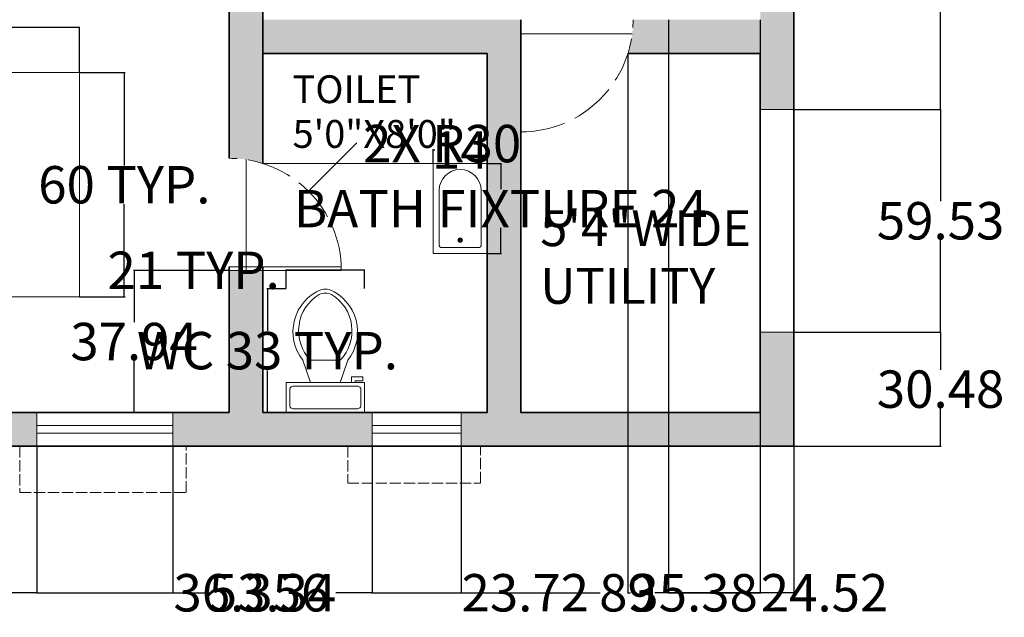
# Model space of a CAD drawing. Units: inches. Extents: x 143 to 746, y -392 to 145.
# Tile 4 of 6: x 473 to 736, y -392 to -233. Entities that reach past the tile are written whole.
import ezdxf

# ---------------------------------------------------------------- set-up
doc = ezdxf.new("R2010")
doc.units = ezdxf.units.IN
doc.header["$MEASUREMENT"] = 0
doc.linetypes.add('ACAD_ISO02W100', pattern=[15, 12, -3])
for name, color, linetype, lineweight in [('A-ANNO-DIMS', 2, 'Continuous', 18), ('A-AREA-IDEN', 7, 'Continuous', 20), ('A-DOOR', 3, 'Continuous', 18), ('A-DOOR-SWNG', 3, 'ACAD_ISO02W100', 13), ('A-FLOR-FIXT', 9, 'Continuous', 18), ('A-FURN', 8, 'Continuous', 18), ('A-GLAZ', 4, 'Continuous', 18), ('A-GLAZ-OVHD', 4, 'ACAD_ISO02W100', 13), ('A-WALL', 7, 'Continuous', 35)]:
    doc.layers.add(name, color=color, linetype=linetype, lineweight=lineweight)
doc.layers.add('A-WALL-PATT', color=252, linetype='Continuous', lineweight=13, true_color=0x939598)
doc.styles.get("Standard").update_dxf_attribs({"font": 'arial.ttf'})
doc.dimstyles.get("Standard").update_dxf_attribs({"dimtxt": 10, "dimasz": 0.18, "dimexe": 0.18, "dimexo": 0.0625, "dimgap": 0.09, "dimtad": 0, "dimtih": 1, "dimtoh": 1, "dimdec": 0, "dimzin": 0, "dimdsep": 46, "dimlunit": 3, "dimtxsty": 'Standard', "dimcen": 0.09, "dimadec": 0, "dimazin": 0, "dimtfac": 1, "dimtdec": 0, "dimtofl": 0, "dimtmove": 0, "dimatfit": 3, "dimfxl": 1, "dimtolj": 1, "dimtzin": 0, "dimarcsym": 0})

# ---------------------------------------------------------------- blocks, each defined once
blk = doc.blocks.new('Toilet - top')
for p, q in [((9.5, -6), (9.5, -2)), ((-10, -8.5), (-8, -8.5)), ((-10, -9.5), (-10, -8.5)), ((-7, -9.5), (-10, -9.5)), ((-8, -8.5), (-8, -8)), ((-7, -8), (-7, -9.5)), ((-4, -8), (-6, -14)), ((4, -8), (6, -14)), ((4, -14), (-4, -14))]:
    blk.add_line(p, q)
blk.add_lwpolyline([(10.5, -8), (10.5, 0), (-10.5, 0), (-10.5, -8)], close=True)
for points in [[(-9.5, -2), (-9.5, -6)], [(8.5, -1), (-8.5, -1)], [(-8.5, -7), (8.5, -7)]]:
    blk.add_lwpolyline(points)
for centre, radius, start, end in [((-8.62, -1.88), 0.884, 81.8699, 188.1301), ((8.62, -1.88), 0.884, 351.8699, 98.1301), ((-8.62, -6.12), 0.884, 171.8699, 278.1301), ((8.62, -6.12), 0.884, 261.8699, 8.1301), ((3.52, -21.58), 12.17, 141.4691, 247.9714), ((4.2, -21.82), 11.33, 136.3677, 238.9468), ((-3.52, -21.58), 12.17, 292.0284, 38.5307), ((-4.2, -21.82), 11.33, 301.053, 43.6321), ((0, -27.88), 4, 245.7318, 294.2682), ((0, -29), 4, 254.8605, 285.1395)]:
    blk.add_arc(centre, radius, start, end)
blk = doc.blocks.new('Bath Tub - 26 x 60 in.')
for p, q in [((8, -18), (10, -18)), ((9, -17), (9, -19))]:
    blk.add_line(p, q)
blk.add_lwpolyline([(0, -36), (0, 0), (60, 0), (60, -36)], close=True)
for points in [[(4, -30), (4, -6)], [(6, -4), (42, -4)], [(42, -32), (6, -32)]]:
    blk.add_lwpolyline(points)
for radius in [1.5, 1]:
    blk.add_circle((9, -18), radius)
for centre, radius, start, end in [((5.75, -5.75), 1.77, 81.8699, 188.1301), ((42, -18), 14, 270, 90), ((5.75, -30.25), 1.77, 171.8699, 278.1301)]:
    blk.add_arc(centre, radius, start, end)
blk = doc.blocks.new('Bed - Queen')
for p, q in [((0, -80.00003), (0, 0)), ((0, 0), (59.99999, 0)), ((59.99999, 0), (59.99999, -80.00003)), ((7.99999, -1.2), (28.79998, -1.2)), ((7.99999, -14.4), (7.99999, -1.2)), ((28.79998, -1.2), (28.79998, -14.4)), ((31.19999, -1.2), (51.99999, -1.2)), ((31.19999, -14.4), (31.19999, -1.2)), ((51.99999, -1.2), (51.99999, -16.4)), ((0, -14.4), (44.8, -14.4)), ((59.99999, -29.6), (44.8, -14.4)), ((44.8, -14.4), (44.8, -29.6)), ((44.8, -16.8), (0, -16.8)), ((51.99999, -16.4), (46.79936, -16.4)), ((44.8, -29.6), (59.99999, -29.6)), ((59.99999, -80.00003), (0, -80.00003))]:
    blk.add_line(p, q)
blk = doc.blocks.new('*D12')
at = {"layer": 'A-ANNO-DIMS', "color": 0, "lineweight": -2, "transparency": 16777216}
for p, q in [((369.19, -220.67), (369.19, -225.34)), ((399.54, -220.67), (399.54, -225.34)), ((369.37, -225.16), (399.36, -225.16)), ((399.54, -225.16), (399.72, -225.16))]:
    blk.add_line(p, q, dxfattribs=at)
at = {"layer": 'A-ANNO-DIMS', "color": 0, "transparency": 16777216}
for points in [[(369.37, -225.13), (369.37, -225.19), (369.19, -225.16)], [(399.36, -225.13), (399.36, -225.19), (399.54, -225.16)]]:
    blk.add_solid(points, dxfattribs=at)
at = {"layer": 'Defpoints', "color": 0, "transparency": 16777216}
for p in [(369.19, -220.61), (399.54, -220.61), (399.54, -225.16)]:
    blk.add_point(p, dxfattribs=at)
at = {"layer": 'A-ANNO-DIMS', "color": 0, "transparency": 16777216, "insert": (459.12, -225.16), "char_height": 10, "attachment_point": 5}
blk.add_mtext('\\A1;BATH FIXTURE 30', dxfattribs=at)
blk = doc.blocks.new('*D14')
at = {"layer": 'A-ANNO-DIMS', "color": 0, "lineweight": -2, "transparency": 16777216}
for p, q in [((597.6, -271.05), (601.33, -271.05)), ((601.15, -271.23), (601.15, -277.9)), ((601.15, -294.96), (601.15, -288.29)), ((597.6, -295.14), (601.33, -295.14))]:
    blk.add_line(p, q, dxfattribs=at)
at = {"layer": 'A-ANNO-DIMS', "color": 0, "transparency": 16777216}
for points in [[(601.12, -271.23), (601.18, -271.23), (601.15, -271.05)], [(601.12, -294.96), (601.18, -294.96), (601.15, -295.14)]]:
    blk.add_solid(points, dxfattribs=at)
at = {"layer": 'Defpoints', "color": 0, "transparency": 16777216}
for p in [(597.54, -271.05), (601.15, -271.05), (597.54, -295.14)]:
    blk.add_point(p, dxfattribs=at)
at = {"layer": 'A-ANNO-DIMS', "color": 0, "transparency": 16777216, "insert": (601.15, -283.1), "char_height": 10, "attachment_point": 5}
blk.add_mtext('\\A1;BATH FIXTURE 24', dxfattribs=at)
blk = doc.blocks.new('*D15')
at = {"layer": 'A-ANNO-DIMS', "color": 0, "lineweight": -2, "transparency": 16777216}
for p, q in [((583.08, -270.99), (583.08, -267.25)), ((583.26, -267.43), (583.55, -267.43)), ((597.36, -267.43), (597.07, -267.43)), ((597.54, -270.99), (597.54, -267.25))]:
    blk.add_line(p, q, dxfattribs=at)
at = {"layer": 'A-ANNO-DIMS', "color": 0, "transparency": 16777216}
for points in [[(583.26, -267.4), (583.26, -267.46), (583.08, -267.43)], [(597.36, -267.4), (597.36, -267.46), (597.54, -267.43)]]:
    blk.add_solid(points, dxfattribs=at)
at = {"layer": 'Defpoints', "color": 0, "transparency": 16777216}
for p in [(583.08, -267.43), (583.08, -271.05), (597.54, -271.05)]:
    blk.add_point(p, dxfattribs=at)
at = {"layer": 'A-ANNO-DIMS', "color": 0, "transparency": 16777216, "insert": (590.31, -267.43), "char_height": 10, "attachment_point": 5}
blk.add_mtext('\\A1;14', dxfattribs=at)
blk = doc.blocks.new('*D22')
at = {"layer": 'A-ANNO-DIMS', "color": 0, "lineweight": -2, "transparency": 16777216}
for p, q in [((543.7, -304.56), (538.62, -304.56)), ((538.8, -304.74), (538.8, -315.82)), ((538.8, -337.43), (538.8, -326.35)), ((543.7, -337.61), (538.62, -337.61))]:
    blk.add_line(p, q, dxfattribs=at)
at = {"layer": 'A-ANNO-DIMS', "color": 0, "transparency": 16777216}
for points in [[(538.77, -304.74), (538.83, -304.74), (538.8, -304.56)], [(538.77, -337.43), (538.83, -337.43), (538.8, -337.61)]]:
    blk.add_solid(points, dxfattribs=at)
at = {"layer": 'Defpoints', "color": 0, "transparency": 16777216}
for p in [(543.76, -304.56), (538.8, -337.61), (543.76, -337.61)]:
    blk.add_point(p, dxfattribs=at)
at = {"layer": 'A-ANNO-DIMS', "color": 0, "transparency": 16777216, "insert": (538.8, -321.08), "char_height": 10, "attachment_point": 5}
blk.add_mtext('\\A1;WC 33 TYP.', dxfattribs=at)
blk = doc.blocks.new('*D23')
at = {"layer": 'A-ANNO-DIMS', "color": 0, "lineweight": -2, "transparency": 16777216}
for p, q in [((543.76, -299.6), (543.58, -299.6)), ((543.76, -304.5), (543.76, -299.42)), ((564.58, -299.6), (543.94, -299.6)), ((564.76, -304.5), (564.76, -299.42))]:
    blk.add_line(p, q, dxfattribs=at)
at = {"layer": 'A-ANNO-DIMS', "color": 0, "transparency": 16777216}
for points in [[(543.94, -299.57), (543.94, -299.63), (543.76, -299.6)], [(564.58, -299.57), (564.58, -299.63), (564.76, -299.6)]]:
    blk.add_solid(points, dxfattribs=at)
at = {"layer": 'Defpoints', "color": 0, "transparency": 16777216}
for p in [(543.76, -299.6), (543.76, -304.56), (564.76, -304.56)]:
    blk.add_point(p, dxfattribs=at)
at = {"layer": 'A-ANNO-DIMS', "color": 0, "transparency": 16777216, "insert": (519.07, -299.6), "char_height": 10, "attachment_point": 5}
blk.add_mtext('\\A1;21 TYP.', dxfattribs=at)
blk = doc.blocks.new('*D24')
at = {"layer": 'A-ANNO-DIMS', "color": 0, "lineweight": -2, "transparency": 16777216}
for p, q in [((408.54, -234.73), (408.36, -234.73)), ((408.54, -246.67), (408.54, -234.55)), ((488.36, -234.73), (408.72, -234.73)), ((488.54, -246.67), (488.54, -234.55))]:
    blk.add_line(p, q, dxfattribs=at)
at = {"layer": 'A-ANNO-DIMS', "color": 0, "transparency": 16777216}
for points in [[(408.72, -234.7), (408.72, -234.76), (408.54, -234.73)], [(488.36, -234.7), (488.36, -234.76), (488.54, -234.73)]]:
    blk.add_solid(points, dxfattribs=at)
at = {"layer": 'Defpoints', "color": 0, "transparency": 16777216}
for p in [(408.54, -234.73), (408.54, -246.73), (488.54, -246.73)]:
    blk.add_point(p, dxfattribs=at)
at = {"layer": 'A-ANNO-DIMS', "color": 0, "transparency": 16777216, "insert": (340.86, -234.73), "char_height": 10, "attachment_point": 5}
blk.add_mtext('\\A1;QUEEN BED 80 TYP.', dxfattribs=at)
blk = doc.blocks.new('*D25')
at = {"layer": 'A-ANNO-DIMS', "color": 0, "lineweight": -2, "transparency": 16777216}
for p, q in [((488.6, -246.73), (500.72, -246.73)), ((500.54, -246.91), (500.54, -271.54)), ((500.54, -306.55), (500.54, -281.93)), ((488.6, -306.73), (500.72, -306.73))]:
    blk.add_line(p, q, dxfattribs=at)
at = {"layer": 'A-ANNO-DIMS', "color": 0, "transparency": 16777216}
for points in [[(500.51, -246.91), (500.57, -246.91), (500.54, -246.73)], [(500.51, -306.55), (500.57, -306.55), (500.54, -306.73)]]:
    blk.add_solid(points, dxfattribs=at)
at = {"layer": 'Defpoints', "color": 0, "transparency": 16777216}
for p in [(488.54, -246.73), (500.54, -246.73), (488.54, -306.73)]:
    blk.add_point(p, dxfattribs=at)
at = {"layer": 'A-ANNO-DIMS', "color": 0, "transparency": 16777216, "insert": (500.54, -276.73), "char_height": 10, "attachment_point": 5}
blk.add_mtext('\\A1;60 TYP.', dxfattribs=at)
blk = doc.blocks.new('*D38')
at = {"layer": 'A-ANNO-DIMS', "color": 0, "lineweight": -2, "transparency": 16777216}
for p, q in [((388.66, -346.67), (388.66, -385.98)), ((477.13, -346.67), (477.13, -385.98)), ((388.84, -385.8), (415.92, -385.8)), ((476.95, -385.8), (449.86, -385.8))]:
    blk.add_line(p, q, dxfattribs=at)
at = {"layer": 'A-ANNO-DIMS', "color": 0, "transparency": 16777216}
for points in [[(388.84, -385.77), (388.84, -385.83), (388.66, -385.8)], [(476.95, -385.77), (476.95, -385.83), (477.13, -385.8)]]:
    blk.add_solid(points, dxfattribs=at)
at = {"layer": 'Defpoints', "color": 0, "transparency": 16777216}
for p in [(388.66, -346.61), (477.13, -346.61), (477.13, -385.8)]:
    blk.add_point(p, dxfattribs=at)
at = {"layer": 'A-ANNO-DIMS', "color": 0, "transparency": 16777216, "insert": (432.89, -385.8), "char_height": 10, "attachment_point": 5}
blk.add_mtext('\\A1;88.47', dxfattribs=at)
blk = doc.blocks.new('*D39')
at = {"layer": 'A-ANNO-DIMS', "color": 0, "lineweight": -2, "transparency": 16777216}
for p, q in [((477.13, -346.67), (477.13, -385.98)), ((513.48, -346.67), (513.48, -385.98)), ((477.31, -385.8), (513.3, -385.8)), ((513.48, -385.8), (513.66, -385.8))]:
    blk.add_line(p, q, dxfattribs=at)
at = {"layer": 'A-ANNO-DIMS', "color": 0, "transparency": 16777216}
for points in [[(477.31, -385.77), (477.31, -385.83), (477.13, -385.8)], [(513.3, -385.77), (513.3, -385.83), (513.48, -385.8)]]:
    blk.add_solid(points, dxfattribs=at)
at = {"layer": 'Defpoints', "color": 0, "transparency": 16777216}
for p in [(477.13, -346.61), (513.48, -346.61), (513.48, -385.8)]:
    blk.add_point(p, dxfattribs=at)
at = {"layer": 'A-ANNO-DIMS', "color": 0, "transparency": 16777216, "insert": (534.5, -385.8), "char_height": 10, "attachment_point": 5}
blk.add_mtext('\\A1;36.356', dxfattribs=at)
blk = doc.blocks.new('*D40')
at = {"layer": 'A-ANNO-DIMS', "color": 0, "lineweight": -2, "transparency": 16777216}
for p, q in [((513.48, -346.67), (513.48, -385.98)), ((566.83, -346.67), (566.83, -385.98)), ((513.66, -385.8), (523.21, -385.8)), ((566.65, -385.8), (557.1, -385.8))]:
    blk.add_line(p, q, dxfattribs=at)
at = {"layer": 'A-ANNO-DIMS', "color": 0, "transparency": 16777216}
for points in [[(513.66, -385.77), (513.66, -385.83), (513.48, -385.8)], [(566.65, -385.77), (566.65, -385.83), (566.83, -385.8)]]:
    blk.add_solid(points, dxfattribs=at)
at = {"layer": 'Defpoints', "color": 0, "transparency": 16777216}
for p in [(513.48, -346.61), (566.83, -346.61), (566.83, -385.8)]:
    blk.add_point(p, dxfattribs=at)
at = {"layer": 'A-ANNO-DIMS', "color": 0, "transparency": 16777216, "insert": (540.15, -385.8), "char_height": 10, "attachment_point": 5}
blk.add_mtext('\\A1;53.34', dxfattribs=at)
blk = doc.blocks.new('*D41')
at = {"layer": 'A-ANNO-DIMS', "color": 0, "lineweight": -2, "transparency": 16777216}
for p, q in [((566.83, -346.67), (566.83, -385.98)), ((590.54, -346.67), (590.54, -385.98)), ((567.01, -385.8), (590.36, -385.8)), ((590.54, -385.8), (590.72, -385.8))]:
    blk.add_line(p, q, dxfattribs=at)
at = {"layer": 'A-ANNO-DIMS', "color": 0, "transparency": 16777216}
for points in [[(567.01, -385.77), (567.01, -385.83), (566.83, -385.8)], [(590.36, -385.77), (590.36, -385.83), (590.54, -385.8)]]:
    blk.add_solid(points, dxfattribs=at)
at = {"layer": 'Defpoints', "color": 0, "transparency": 16777216}
for p in [(566.83, -346.61), (590.54, -346.61), (590.54, -385.8)]:
    blk.add_point(p, dxfattribs=at)
at = {"layer": 'A-ANNO-DIMS', "color": 0, "transparency": 16777216, "insert": (607.72, -385.8), "char_height": 10, "attachment_point": 5}
blk.add_mtext('\\A1;23.72', dxfattribs=at)
blk = doc.blocks.new('*D42')
at = {"layer": 'A-ANNO-DIMS', "color": 0, "lineweight": -2, "transparency": 16777216}
for p, q in [((590.54, -346.67), (590.54, -385.98)), ((679.54, -346.67), (679.54, -385.98)), ((590.72, -385.8), (627.77, -385.8)), ((679.36, -385.8), (642.31, -385.8))]:
    blk.add_line(p, q, dxfattribs=at)
at = {"layer": 'A-ANNO-DIMS', "color": 0, "transparency": 16777216}
for points in [[(590.72, -385.77), (590.72, -385.83), (590.54, -385.8)], [(679.36, -385.77), (679.36, -385.83), (679.54, -385.8)]]:
    blk.add_solid(points, dxfattribs=at)
at = {"layer": 'Defpoints', "color": 0, "transparency": 16777216}
for p in [(590.54, -346.61), (679.54, -346.61), (679.54, -385.8)]:
    blk.add_point(p, dxfattribs=at)
at = {"layer": 'A-ANNO-DIMS', "color": 0, "transparency": 16777216, "insert": (635.04, -385.8), "char_height": 10, "attachment_point": 5}
blk.add_mtext('\\A1;89', dxfattribs=at)
blk = doc.blocks.new('*D61')
at = {"layer": 'A-ANNO-DIMS', "color": 0, "lineweight": -2, "transparency": 16777216}
for p, q in [((679.6, -187.05), (718.91, -187.05)), ((718.73, -187.23), (718.73, -216.63)), ((718.73, -256.42), (718.73, -227.02)), ((679.6, -256.6), (718.91, -256.6))]:
    blk.add_line(p, q, dxfattribs=at)
at = {"layer": 'A-ANNO-DIMS', "color": 0, "transparency": 16777216}
for points in [[(718.7, -187.23), (718.76, -187.23), (718.73, -187.05)], [(718.7, -256.42), (718.76, -256.42), (718.73, -256.6)]]:
    blk.add_solid(points, dxfattribs=at)
at = {"layer": 'Defpoints', "color": 0, "transparency": 16777216}
for p in [(679.54, -187.05), (679.54, -256.6), (718.73, -256.6)]:
    blk.add_point(p, dxfattribs=at)
at = {"layer": 'A-ANNO-DIMS', "color": 0, "transparency": 16777216, "insert": (718.73, -221.82), "char_height": 10, "attachment_point": 5}
blk.add_mtext('\\A1;69.55', dxfattribs=at)
blk = doc.blocks.new('*D62')
at = {"layer": 'A-ANNO-DIMS', "color": 0, "lineweight": -2, "transparency": 16777216}
for p, q in [((679.6, -256.6), (718.91, -256.6)), ((718.73, -256.78), (718.73, -281.16)), ((718.73, -315.95), (718.73, -291.56)), ((679.6, -316.13), (718.91, -316.13))]:
    blk.add_line(p, q, dxfattribs=at)
at = {"layer": 'A-ANNO-DIMS', "color": 0, "transparency": 16777216}
for points in [[(718.7, -256.78), (718.76, -256.78), (718.73, -256.6)], [(718.7, -315.95), (718.76, -315.95), (718.73, -316.13)]]:
    blk.add_solid(points, dxfattribs=at)
at = {"layer": 'Defpoints', "color": 0, "transparency": 16777216}
for p in [(679.54, -256.6), (679.54, -316.13), (718.73, -316.13)]:
    blk.add_point(p, dxfattribs=at)
at = {"layer": 'A-ANNO-DIMS', "color": 0, "transparency": 16777216, "insert": (718.73, -286.36), "char_height": 10, "attachment_point": 5}
blk.add_mtext('\\A1;59.53', dxfattribs=at)
blk = doc.blocks.new('*D63')
at = {"layer": 'A-ANNO-DIMS', "color": 0, "lineweight": -2, "transparency": 16777216}
for p, q in [((679.6, -316.13), (718.91, -316.13)), ((718.73, -316.31), (718.73, -326.17)), ((718.73, -346.43), (718.73, -336.57)), ((679.6, -346.61), (718.91, -346.61))]:
    blk.add_line(p, q, dxfattribs=at)
at = {"layer": 'A-ANNO-DIMS', "color": 0, "transparency": 16777216}
for points in [[(718.7, -316.31), (718.76, -316.31), (718.73, -316.13)], [(718.7, -346.43), (718.76, -346.43), (718.73, -346.61)]]:
    blk.add_solid(points, dxfattribs=at)
at = {"layer": 'Defpoints', "color": 0, "transparency": 16777216}
for p in [(679.54, -316.13), (679.54, -346.61), (718.73, -346.61)]:
    blk.add_point(p, dxfattribs=at)
at = {"layer": 'A-ANNO-DIMS', "color": 0, "transparency": 16777216, "insert": (718.73, -331.37), "char_height": 10, "attachment_point": 5}
blk.add_mtext('\\A1;30.48', dxfattribs=at)
blk = doc.blocks.new('*D64')
at = {"layer": 'A-ANNO-DIMS', "color": 0, "lineweight": -2, "transparency": 16777216}
for p, q in [((646.02, -232.67), (646.02, -385.98)), ((670.54, -232.67), (670.54, -385.98)), ((646.2, -385.8), (670.36, -385.8)), ((670.54, -385.8), (670.72, -385.8))]:
    blk.add_line(p, q, dxfattribs=at)
at = {"layer": 'A-ANNO-DIMS', "color": 0, "transparency": 16777216}
for points in [[(646.2, -385.77), (646.2, -385.83), (646.02, -385.8)], [(670.36, -385.77), (670.36, -385.83), (670.54, -385.8)]]:
    blk.add_solid(points, dxfattribs=at)
at = {"layer": 'Defpoints', "color": 0, "transparency": 16777216}
for p in [(646.02, -232.61), (670.54, -232.61), (670.54, -385.8)]:
    blk.add_point(p, dxfattribs=at)
at = {"layer": 'A-ANNO-DIMS', "color": 0, "transparency": 16777216, "insert": (687.71, -385.8), "char_height": 10, "attachment_point": 5}
blk.add_mtext('\\A1;24.52', dxfattribs=at)
blk = doc.blocks.new('*D73')
at = {"layer": 'A-ANNO-DIMS', "color": 0, "lineweight": -2, "transparency": 16777216}
for p, q in [((528.48, -299.67), (502.96, -299.67)), ((503.14, -299.85), (503.14, -313.44)), ((503.14, -337.43), (503.14, -323.84)), ((528.48, -337.61), (502.96, -337.61))]:
    blk.add_line(p, q, dxfattribs=at)
at = {"layer": 'A-ANNO-DIMS', "color": 0, "transparency": 16777216}
for points in [[(503.11, -299.85), (503.17, -299.85), (503.14, -299.67)], [(503.11, -337.43), (503.17, -337.43), (503.14, -337.61)]]:
    blk.add_solid(points, dxfattribs=at)
at = {"layer": 'Defpoints', "color": 0, "transparency": 16777216}
for p in [(503.14, -299.67), (528.54, -299.67), (528.54, -337.61)]:
    blk.add_point(p, dxfattribs=at)
at = {"layer": 'A-ANNO-DIMS', "color": 0, "transparency": 16777216, "insert": (503.14, -318.64), "char_height": 10, "attachment_point": 5}
blk.add_mtext('\\A1;37.94', dxfattribs=at)
blk = doc.blocks.new('*D74')
at = {"layer": 'A-ANNO-DIMS', "color": 0, "lineweight": -2, "transparency": 16777216}
for p, q in [((635.16, -241.67), (635.16, -385.98)), ((670.54, -241.67), (670.54, -385.98)), ((635.34, -385.8), (635.88, -385.8)), ((670.36, -385.8), (669.82, -385.8))]:
    blk.add_line(p, q, dxfattribs=at)
at = {"layer": 'A-ANNO-DIMS', "color": 0, "transparency": 16777216}
for points in [[(635.34, -385.77), (635.34, -385.83), (635.16, -385.8)], [(670.36, -385.77), (670.36, -385.83), (670.54, -385.8)]]:
    blk.add_solid(points, dxfattribs=at)
at = {"layer": 'Defpoints', "color": 0, "transparency": 16777216}
for p in [(635.16, -241.61), (670.54, -241.61), (670.54, -385.8)]:
    blk.add_point(p, dxfattribs=at)
at = {"layer": 'A-ANNO-DIMS', "color": 0, "transparency": 16777216, "insert": (652.85, -385.8), "char_height": 10, "attachment_point": 5}
blk.add_mtext('\\A1;35.38', dxfattribs=at)
blk = doc.blocks.new('*D76')
at = {"layer": 'A-ANNO-DIMS', "color": 0, "lineweight": -2, "transparency": 16777216}
for p, q in [((562.48, -265.73), (549.88, -278.33)), ((562.66, -265.73), (562.48, -265.73)), ((528.45, -299.67), (528.63, -299.67)), ((528.54, -299.76), (528.54, -299.58))]:
    blk.add_line(p, q, dxfattribs=at)
at = {"layer": 'A-ANNO-DIMS', "color": 0, "transparency": 16777216}
blk.add_solid([(549.86, -278.31), (549.9, -278.35), (549.75, -278.45)], dxfattribs=at)
at = {"layer": 'Defpoints', "color": 0, "transparency": 16777216}
for p in [(549.75, -278.45), (528.54, -299.67)]:
    blk.add_point(p, dxfattribs=at)
at = {"layer": 'A-ANNO-DIMS', "color": 0, "transparency": 16777216, "insert": (585.51, -265.73), "char_height": 10, "attachment_point": 5}
blk.add_mtext('\\A1;2X R30', dxfattribs=at)

msp = doc.modelspace()

# ---------------------------------------------------------------- hatches: boundary and pattern name
at = {"layer": 'A-WALL-PATT'}
h = msp.add_hatch(color=256, dxfattribs=at)
h.dxf.hatch_style = 1
h.paths.add_polyline_path([(198.538, 19.3924), (257.4275, 19.3924), (257.4275, 28.3924), (189.538, 28.3924), (189.538, -95.6731, -0.06325422), (198.538, -96.8162)])
h.paths.add_polyline_path([(339.538, 66.969), (471.538, 66.969), (472.538, 66.969), (472.538, 31.3924), (472.538, 6.969), (451.2296, 6.969), (451.2296, -2.031), (472.538, -2.031), (472.538, -82.6076), (544.538, -82.6076), (544.538, -38.6894), (535.538, -38.6894), (535.538, -73.6076), (481.538, -73.6076), (481.538, 22.3924), (498.7149, 22.3924), (498.7149, 31.3924), (481.538, 31.3924), (481.538, 66.969), (481.538, 113.4779), (471.538, 113.4779), (471.538, 75.969), (339.538, 75.969), (339.538, 113.4779), (330.538, 113.4779), (330.538, 66.969), (330.538, 28.3924), (293.6446, 28.3924), (293.6446, 19.3924), (330.538, 19.3924), (330.538, 6.969), (330.538, -2.031), (364.5099, -2.031), (364.5099, 6.969), (339.538, 6.969)])
h.paths.add_polyline_path([(570.63, 31.3924), (544.538, 31.3924), (524.7988, 31.3924), (524.7988, 22.3924), (535.538, 22.3924), (535.538, -9.9696, -0.0761882), (544.538, -8.6878), (544.538, 22.3924), (570.63, 22.3924)])
h.paths.add_polyline_path([(679.538, 31.3924), (618.768, 31.3924), (618.768, 22.3924), (670.538, 22.3924), (670.538, -54.5218), (679.538, -54.5218)])
h.paths.add_polyline_path([(679.538, -90.0753), (670.538, -90.0753), (670.538, -121.6076), (537.538, -121.6076), (528.538, -121.6076), (528.538, -130.6076), (537.538, -130.6076), (670.538, -130.6076), (670.538, -150.8923), (679.538, -150.8923)])
h.paths.add_polyline_path([(679.538, -187.0502), (670.538, -187.0502), (670.538, -232.6076), (636.538, -232.6076, -0.07632083), (635.1562, -241.6076), (670.538, -241.6076), (670.538, -256.599), (679.538, -256.599)])
h.paths.add_polyline_path([(606.538, -232.6076), (537.538, -232.6076), (537.538, -241.6076), (597.538, -241.6076), (597.538, -337.6076), (590.545, -337.6076), (590.545, -346.6076), (679.538, -346.6076), (679.538, -316.1251), (670.538, -316.1251), (670.538, -337.6076), (606.538, -337.6076)])
h.paths.add_polyline_path([(537.538, -181.6076), (537.538, -172.6076), (528.538, -172.6076), (528.538, -209.005), (528.538, -269.6672, -0.07632083), (537.538, -271.0491)])
h.paths.add_polyline_path([(566.8252, -337.6076), (537.538, -337.6076), (537.538, -299.6672), (528.538, -299.6672), (528.538, -337.6076), (513.484, -337.6076), (513.484, -346.6076), (566.8252, -346.6076)])
h.paths.add_polyline_path([(477.1278, -337.6076), (408.538, -337.6076), (408.538, -229.6076), (408.538, -181.6076), (493.5793, -181.6076, -0.06316411), (492.538, -172.6076), (399.538, -172.6076), (399.538, -229.6076), (399.538, -337.6076), (388.659, -337.6076), (388.659, -346.6076), (477.1278, -346.6076)])
h.paths.add_polyline_path([(364.4504, -337.6076), (339.538, -337.6076), (339.538, -301.3371), (330.538, -301.3371), (330.538, -337.6076), (307.2736, -337.6076), (307.2736, -346.6076), (364.4504, -346.6076)])
h.paths.add_polyline_path([(339.538, -229.6076), (399.538, -229.6076), (399.538, -220.6076), (369.1898, -220.6076), (330.538, -220.6076), (330.538, -271.2389, -0.07612824), (339.538, -272.6672)])
h.paths.add_polyline_path([(271.3704, -337.6076), (198.538, -337.6076), (198.538, -181.6076), (339.538, -181.6076), (339.538, -172.6076), (198.538, -172.6076), (198.538, -131.6731), (189.538, -131.6731), (189.538, -346.6076), (271.3704, -346.6076)])

# ---------------------------------------------------------------- linework, layer by layer
at = {"layer": 'A-DOOR'}
for p, q in [((606.538, -232.6076), (606.538, -262.6076)), ((636.298, -236.3952), (606.538, -236.3952)), ((533.1427, -299.6672), (533.1427, -270.0227)), ((528.538, -299.6672), (528.538, -298.6672)), ((528.538, -298.6672), (558.538, -298.6672)), ((528.538, -299.6672), (558.538, -299.6672))]:
    msp.add_line(p, q, dxfattribs=at)
at = {"layer": 'A-DOOR-SWNG'}
for centre, start, end in [((606.538, -232.6076), 270, 0), ((528.538, -299.6672), 0, 90)]:
    msp.add_arc(centre, 30, start, end, dxfattribs=at)
at = {"layer": 'A-FLOR-FIXT'}
msp.add_line((537.538, -271.0491), (597.538, -271.0491), dxfattribs=at)
at = {"layer": 'A-GLAZ'}
for p, q in [((670.538, -256.599), (679.538, -256.599)), ((670.538, -316.1251), (679.538, -316.1251)), ((477.1278, -342.1076), (477.1278, -337.6076)), ((477.1278, -337.6076), (477.1278, -346.6076)), ((513.484, -337.6076), (513.484, -346.6076)), ((566.8252, -342.1076), (566.8252, -337.6076)), ((566.8252, -337.6076), (566.8252, -346.6076)), ((590.545, -337.6076), (590.545, -346.6076)), ((513.484, -341.1076), (477.1278, -341.1076)), ((590.545, -341.1076), (566.8252, -341.1076)), ((513.484, -343.1076), (477.1278, -343.1076)), ((590.545, -343.1076), (566.8252, -343.1076))]:
    msp.add_line(p, q, dxfattribs=at)
at = {"layer": 'A-GLAZ-OVHD', "ltscale": 0.25}
for p, q in [((472.5993, -346.6076), (472.5993, -358.9961)), ((517.0583, -358.9961), (517.0583, -346.6076)), ((560.2403, -346.6076), (560.2403, -356.5097)), ((595.7762, -356.5097), (595.7762, -346.6076)), ((560.2403, -356.5097), (595.7762, -356.5097)), ((472.5993, -358.9961), (517.0583, -358.9961))]:
    msp.add_line(p, q, dxfattribs=at)
at = {"layer": 'A-WALL'}
for p, q in [((679.538, -346.6076), (679.538, 31.3924)), ((528.538, -269.6672), (528.538, -172.6076)), ((537.538, -271.0491), (537.538, -181.6076)), ((606.538, -337.6076), (606.538, -232.6076)), ((597.538, -241.6076), (537.538, -241.6076)), ((597.538, -337.6076), (597.538, -241.6076)), ((670.538, -241.6076), (635.1562, -241.6076)), ((670.538, -337.6076), (670.538, -241.6076)), ((679.538, -337.6076), (679.538, -241.6076)), ((528.538, -337.6076), (528.538, -298.6672)), ((537.538, -337.6076), (537.538, -298.6672)), ((408.538, -337.6076), (528.538, -337.6076)), ((537.538, -337.6076), (597.538, -337.6076)), ((606.538, -337.6076), (670.538, -337.6076)), ((189.538, -346.6076), (679.538, -346.6076)), ((408.538, -346.6076), (528.538, -346.6076)), ((537.538, -346.6076), (597.538, -346.6076))]:
    msp.add_line(p, q, dxfattribs=at)

# ---------------------------------------------------------------- block references
at = {"layer": 'A-FLOR-FIXT', "xscale": 0.4015630644271725, "yscale": 0.4015630644271725, "zscale": 0.4015630644271725, "rotation": 90}
msp.add_blockref('Bath Tub - 26 x 60 in.', (583.0818, -295.1428), dxfattribs=at)
at = {"layer": 'A-FLOR-FIXT', "rotation": 180.0000000000007}
msp.add_blockref('Toilet - top', (554.2609, -337.6076), dxfattribs=at)
at = {"layer": 'A-FURN', "rotation": 90}
msp.add_blockref('Bed - Queen', (408.538, -306.7314), dxfattribs=at)

# ---------------------------------------------------------------- texts
at = {"layer": 'A-AREA-IDEN'}
for s, height, p in [('TOILET', 7.44261, (545.5115, -254.9141)), ('5\'0"X8\'0"', 7.44261, (545.5115, -266.87)), ('5\'4"WIDE', 9.58417, (611.7277, -293.1441)), ('UTILITY', 9.58417, (611.7277, -308.5402))]:
    msp.add_text(s, height=height, dxfattribs=at).set_placement(p)

# ---------------------------------------------------------------- dimensions: what is measured, and where the dimension line sits
at = {"layer": 'A-ANNO-DIMS'}
for base, p1, p2, angle, override, picture, middle in [((718.7255, -256.599), (679.538, -187.0502), (679.538, -256.599), 90, {"dimdec": 2, "dimlfac": 1, "dimrnd": 0, "dimzin": 0, "dimdsep": 46, "dimlunit": 2}, '*D61', (718.7255, -221.8246)), ((718.7255, -316.1251), (679.538, -256.599), (679.538, -316.1251), 90, {"dimdec": 2, "dimlfac": 1, "dimrnd": 0, "dimzin": 0, "dimdsep": 46, "dimlunit": 2}, '*D62', (718.7255, -286.3621)), ((583.0818, -267.435), (597.538, -271.0491), (583.0818, -271.0491), 180, {"dimdec": 0, "dimlfac": 1, "dimrnd": 0, "dimzin": 0, "dimdsep": 46, "dimlunit": 2}, '*D15', (590.3099, -267.435)), ((503.138, -299.6672), (528.538, -337.6076), (528.538, -299.6672), 90, {"dimdec": 2, "dimlfac": 1, "dimrnd": 0, "dimzin": 0, "dimdsep": 46, "dimlunit": 2}, '*D73', (503.138, -318.6374)), ((718.7255, -346.6076), (679.538, -316.1251), (679.538, -346.6076), 90, {"dimdec": 2, "dimlfac": 1, "dimrnd": 0, "dimzin": 0, "dimdsep": 46, "dimlunit": 2}, '*D63', (718.7255, -331.3664))]:
    dim = msp.add_linear_dim(base=base, p1=p1, p2=p2, angle=angle, dimstyle='Standard', override=override, dxfattribs=at)
    dim.commit()
    dim.dimension.update_dxf_attribs({"geometry": picture, "text_midpoint": middle})
dim = msp.add_linear_dim(base=(399.538, -225.1598), p1=(369.1898, -220.6076), p2=(399.538, -220.6076), text='BATH FIXTURE <>', dimstyle='Standard', override={"dimdec": 0, "dimlfac": 1, "dimrnd": 0, "dimzin": 0, "dimdsep": 46, "dimlunit": 2}, dxfattribs=at)
dim.commit()
dim.dimension.update_dxf_attribs({"geometry": '*D12', "text_midpoint": (459.1225, -225.1598)})
for base, p1, p2, angle, text, picture, middle in [((408.538, -234.7314), (488.5381, -246.7314), (408.538, -246.7314), 180, 'QUEEN BED <> TYP.', '*D24', (340.8567, -234.7314)), ((500.5381, -246.7314), (488.5381, -306.7314), (488.5381, -246.7314), 90, '<> TYP.', '*D25', (500.5381, -276.7314)), ((601.1521, -271.0491), (597.538, -295.1428), (597.538, -271.0491), 90, 'BATH FIXTURE <>', '*D14', (601.1521, -283.0959)), ((543.7609, -299.6044), (564.7609, -304.5614), (543.7609, -304.5614), 180, '<> TYP.', '*D23', (519.0673, -299.6044)), ((538.804, -337.6076), (543.7609, -304.5614), (543.7609, -337.6076), 270, 'WC <> TYP.', '*D22', (538.804, -321.0845))]:
    dim = msp.add_linear_dim(base=base, p1=p1, p2=p2, angle=angle, text=text, dimstyle='Standard', override={"dimdec": 0, "dimlfac": 1, "dimrnd": 0, "dimzin": 0, "dimdsep": 46, "dimlunit": 2}, dxfattribs=at)
    dim.commit()
    dim.dimension.update_dxf_attribs({"geometry": picture, "text_midpoint": middle})
for base, p1, p2, override, picture, middle in [((670.538, -385.7951), (646.0181, -232.6076), (670.538, -232.6076), {"dimdec": 2, "dimlfac": 1, "dimrnd": 0, "dimzin": 0, "dimdsep": 46, "dimlunit": 2}, '*D64', (687.7146, -385.7951)), ((670.538, -385.7951), (635.1562, -241.6076), (670.538, -241.6076), {"dimdec": 2, "dimlfac": 1, "dimrnd": 0, "dimzin": 0, "dimdsep": 46, "dimlunit": 2}, '*D74', (652.8471, -385.7951)), ((477.1278, -385.7951), (388.659, -346.6076), (477.1278, -346.6076), {"dimdec": 2, "dimlfac": 1, "dimrnd": 0, "dimzin": 0, "dimdsep": 46, "dimlunit": 2}, '*D38', (432.8934, -385.7951)), ((513.484, -385.7951), (477.1278, -346.6076), (513.484, -346.6076), {"dimdec": 3, "dimlfac": 1, "dimrnd": 0, "dimzin": 0, "dimdsep": 46, "dimlunit": 2}, '*D39', (534.5043, -385.7951)), ((566.8252, -385.7951), (513.484, -346.6076), (566.8252, -346.6076), {"dimdec": 2, "dimlfac": 1, "dimrnd": 0, "dimzin": 0, "dimdsep": 46, "dimlunit": 2}, '*D40', (540.1546, -385.7951)), ((590.545, -385.7951), (566.8252, -346.6076), (590.545, -346.6076), {"dimdec": 2, "dimlfac": 1, "dimrnd": 0, "dimzin": 0, "dimdsep": 46, "dimlunit": 2}, '*D41', (607.7215, -385.7951)), ((679.538, -385.7951), (590.545, -346.6076), (679.538, -346.6076), {"dimdec": 0, "dimlfac": 1, "dimrnd": 0, "dimzin": 0, "dimdsep": 46, "dimlunit": 2}, '*D42', (635.0415, -385.7951))]:
    dim = msp.add_linear_dim(base=base, p1=p1, p2=p2, dimstyle='Standard', override=override, dxfattribs=at)
    dim.commit()
    dim.dimension.update_dxf_attribs({"geometry": picture, "text_midpoint": middle})
dim = msp.add_radius_dim(center=(528.538, -299.6672), mpoint=(549.7511, -278.4539), text='2X <>', dimstyle='Standard', override={"dimdec": 0, "dimlfac": 1, "dimrnd": 0, "dimzin": 0, "dimdsep": 46, "dimlunit": 2}, dxfattribs=at)
dim.commit()
dim.dimension.update_dxf_attribs({"geometry": '*D76', "text_midpoint": (585.5082, -265.7259), "dimtype": 164})

doc.saveas('drawing.dxf')
